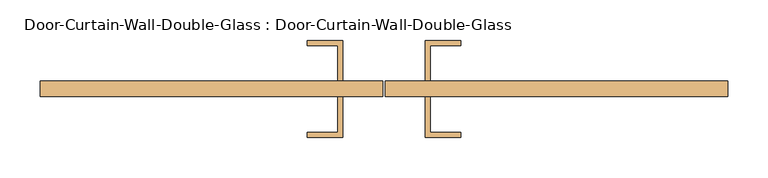
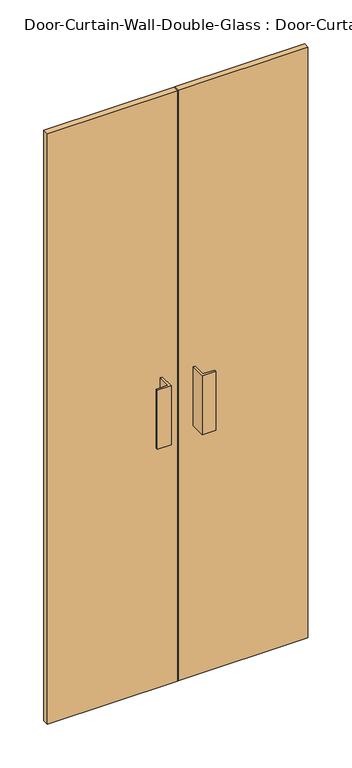
"""IFC4 building model written with IfcOpenShell, lengths in millimetres: door geometry, Door-Curtain-Wall-Double-Glass : Door-Curtain-Wall-Double-Glass."""

from ifc_helpers import new_model, si_unit, frame, origin, origin_with_axes, place, context, project, spatial, polyline, outline, extrude, source, transform, mapped, element, save


def door_curtain_wall_double_glass_door_curtain_wall_double_88735db7(model_context):
    return source(origin(), model_context, "Body", "SweptSolid", [
        extrude(outline(polyline([(425.45, 31.75), (1.5606001, 31.75), (1.5606001, 50.8), (425.45, 50.8), (425.45, 31.75)])), origin_with_axes(), (0.0, 0.0, 1.0), 2038.35),
        extrude(outline(polyline([(-1.6143999, 31.75), (-425.45, 31.75), (-425.45, 50.8), (-1.6143999, 50.8), (-1.6143999, 31.75)])), origin_with_axes(), (0.0, 0.0, 1.0), 2038.35),
        extrude(outline(polyline([(-50.8268999, 101.6), (-50.8268999, 50.8), (-57.1768999, 50.8), (-57.1768999, 95.25), (-95.2768999, 95.25), (-95.2768999, 101.6), (-50.8268999, 101.6)])), frame((0.0, 0.0, 863.6), z_axis=(0.0, 0.0, 1.0), x_axis=(1.0, 0.0, 0.0)), (0.0, 0.0, 1.0), 203.2),
        extrude(outline(polyline([(50.7731001, 101.6), (95.2231001, 101.6), (95.2231001, 95.25), (57.1231001, 95.25), (57.1231001, 50.8), (50.7731001, 50.8), (50.7731001, 101.6)])), frame((0.0, 0.0, 863.6), z_axis=(0.0, 0.0, 1.0), x_axis=(1.0, 0.0, 0.0)), (0.0, 0.0, 1.0), 203.2),
        extrude(outline(polyline([(-50.8268999, -19.05), (-95.2768999, -19.05), (-95.2768999, -12.7), (-57.1768999, -12.7), (-57.1768999, 31.75), (-50.8268999, 31.75), (-50.8268999, -19.05)])), frame((0.0, 0.0, 863.6), z_axis=(0.0, 0.0, 1.0), x_axis=(1.0, 0.0, 0.0)), (0.0, 0.0, 1.0), 203.2),
        extrude(outline(polyline([(50.7731001, -19.05), (50.7731001, 31.75), (57.1231001, 31.75), (57.1231001, -12.7), (95.2231001, -12.7), (95.2231001, -19.05), (50.7731001, -19.05)])), frame((0.0, 0.0, 863.6), z_axis=(0.0, 0.0, 1.0), x_axis=(1.0, 0.0, 0.0)), (0.0, 0.0, 1.0), 203.2),
    ])


if __name__ == "__main__":
    model = new_model("IFC4")
    model_context = context("Model", 3, world=origin())
    ifc_project = project(units=[si_unit("LENGTHUNIT", "METRE", prefix="MILLI")], contexts=[model_context])
    site = spatial("IfcSite", under=ifc_project)
    building = spatial("IfcBuilding", under=site)
    placement = place(None, origin())
    door_curtain_wall_double_glass_door_curtain_wall_double_shape = door_curtain_wall_double_glass_door_curtain_wall_double_88735db7(model_context)
    element("IfcDoor", 1, ObjectType="Door-Curtain-Wall-Double-Glass : Door-Curtain-Wall-Double-Glass", at=placement, inside=building, context=model_context, shape_type="MappedRepresentation", body=[
        mapped(door_curtain_wall_double_glass_door_curtain_wall_double_shape, transform((0.0, 0.0, 0.0), x_axis=(1.0, 0.0, 0.0), y_axis=(0.0, 1.0, 0.0), z_axis=(0.0, 0.0, 1.0))),
    ])
    save(model, "model.ifc")

# Revit data of these elements
# Type "Door-Curtain-Wall-Double-Glass : Door-Curtain-Wall-Double-Glass"
#   Type Mark = "16"
#   Assembly Code = "B2030100"
#   Analytic Construction = "<None>"
#   Width [instance default] = 6' - 0"
#   Thermal Resistance (R) = 10.0000 (h·ft²·°F)/BTU
#   Swing Angle [instance default] = 90.00°
#   Panel Width [instance default] = 3' - 0"
#   Offset = 0' - 2"
#   Heat Transfer Coefficient (U) = 0.1000 BTU/(h·ft²·°F)
#   Define Thermal Properties by = 1
#   Function = 1
#   Door Handle Material = Aluminum
#   Glazing = Glass
#   Visual Light Transmittance = 0
#   Solar Heat Gain Coefficient = 0
#   Construction Type Id = ""
# Element 1 (IfcDoor, "Door-Curtain-Wall-Double-Glass : Door-Curtain-Wall-Double-Glass")
#   Width = 2' - 9 1/2"
#   Panel Width = 1' - 4 3/4"
#   Materials on its faces: "Aluminum", "Glass"
# Materials
#   "Aluminum": class "Metal", colour RGB 247 247 247, transparency 0, Description = "Aluminum 6061", Cost = 0
#   "Glass": class "Glass", colour RGB 0 128 192, transparency 0.75, Description = "Soda Lime Glass", Cost = 0
